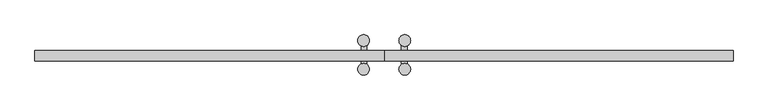
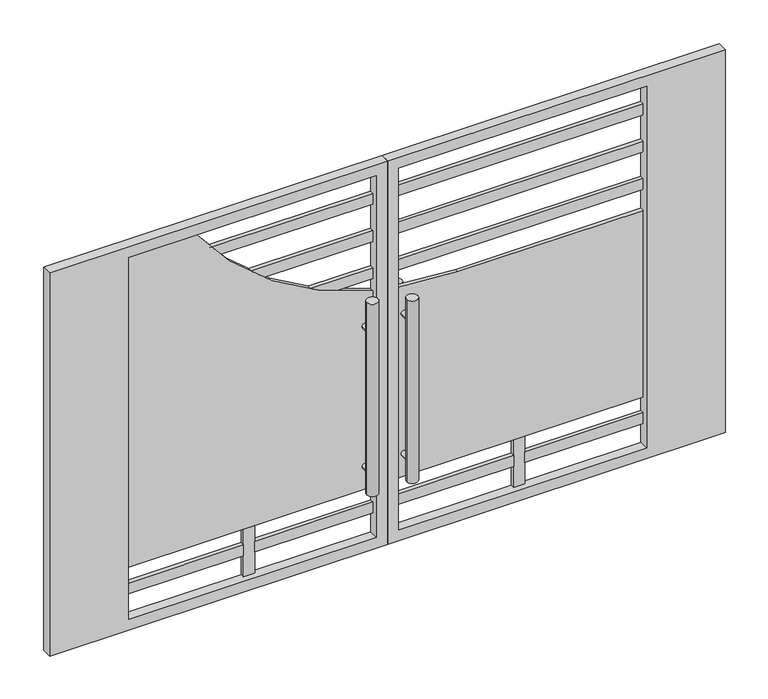
"""IFC4 building model written with IfcOpenShell, lengths in millimetres: proxy geometry."""

from ifc_helpers import new_model, si_unit, point, frame, frame_2d, origin, place, context, project, spatial, polyline, circle_curve, trimmed, segment, composite_curve, outline, extrude, source, transform, mapped, element, save


def generic_models_d903a639(model_context):
    return source(origin(), model_context, "Body", "SweptSolid", [
        extrude(outline(polyline([(0.0, -1524.918066), (0.0, 0.0), (1828.8, 0.0), (1828.8, -1524.918066), (0.0, -1524.918066)]), holes=[polyline([(50.8, -1168.4), (1778.0, -1168.4), (1778.0, -50.8), (50.8, -50.8), (50.8, -1168.4)])]), frame((0.0, -46.0617726, 0.0), z_axis=(0.0, 1.0, 0.0), x_axis=(0.0, 0.0, 1.0)), (0.0, 0.0, 1.0), 46.0617726),
        extrude(outline(polyline([(0.0, 1523.081934), (1828.8, 1523.081934), (1828.8, 0.0), (0.0, 0.0), (0.0, 1523.081934)]), holes=[polyline([(50.8, 1168.4), (50.8, 50.8), (1778.0, 50.8), (1778.0, 1168.4), (50.8, 1168.4)])]), frame((0.0, -46.0617726, 0.0), z_axis=(0.0, 1.0, 0.0), x_axis=(0.0, 0.0, 1.0)), (0.0, 0.0, 1.0), 46.0617726),
        extrude(outline(composite_curve([segment(polyline([(1778.0, -1168.4), (279.4, -1168.4), (279.4, -50.8), (1212.1744192, -50.8)]), True, "CONTINUOUS"), segment(trimmed(circle_curve(frame_2d((2582.6324877, 299.8877691)), 1414.6155764), [point((1212.1744192, -50.8))], [point((1778.0, -863.6))], True, "CARTESIAN"), True, "CONTINUOUS"), segment(polyline([(1778.0, -863.6), (1778.0, -1168.4)]), True, "CONTINUOUS")], self_intersect=False)), frame((0.0, -19.05, 0.0), z_axis=(0.0, 1.0, 0.0), x_axis=(0.0, 0.0, 1.0)), (0.0, 0.0, 1.0), 19.05),
        extrude(outline(composite_curve([segment(polyline([(279.4, 1168.4), (1168.4, 1168.4), (1168.4, 332.8073642)]), True, "CONTINUOUS"), segment(trimmed(circle_curve(frame_2d((2582.6324877, 299.8877691)), 1414.6155764), [point((1168.4, 332.8073642))], [point((1190.1194672, 50.8))], True, "CARTESIAN"), True, "CONTINUOUS"), segment(polyline([(1190.1194672, 50.8), (279.4, 50.8), (279.4, 1168.4)]), True, "CONTINUOUS")], self_intersect=False)), frame((0.0, -19.05, 0.0), z_axis=(0.0, 1.0, 0.0), x_axis=(0.0, 0.0, 1.0)), (0.0, 0.0, 1.0), 19.05),
        extrude(outline(composite_curve([segment(polyline([(1676.4, -50.8), (1676.4, -786.3350015)]), True, "CONTINUOUS"), segment(trimmed(circle_curve(frame_2d((2582.6324877, 299.8877691)), 1414.6155764), [point((1676.4, -786.3350015))], [point((1625.6, -741.8540639))], False, "CARTESIAN"), True, "CONTINUOUS"), segment(polyline([(1625.6, -741.8540639), (1625.6, -50.8), (1676.4, -50.8)]), True, "CONTINUOUS")], self_intersect=False)), frame((0.0, -19.05, 0.0), z_axis=(0.0, 1.0, 0.0), x_axis=(0.0, 0.0, 1.0)), (0.0, 0.0, 1.0), 19.05),
        extrude(outline(polyline([(1171.575, -19.05), (50.8, -19.05), (50.8, 0.0), (1171.575, 0.0), (1171.575, -19.05)])), frame((0.0, 0.0, 1625.6), z_axis=(0.0, 0.0, 1.0), x_axis=(1.0, 0.0, 0.0)), (0.0, 0.0, 1.0), 50.8),
        extrude(outline(composite_curve([segment(polyline([(1498.6, -50.8), (1498.6, -608.963591)]), True, "CONTINUOUS"), segment(trimmed(circle_curve(frame_2d((2582.6324877, 299.8877691)), 1414.6155764), [point((1498.6, -608.963591))], [point((1447.8, -544.6786605))], False, "CARTESIAN"), True, "CONTINUOUS"), segment(polyline([(1447.8, -544.6786605), (1447.8, -50.8), (1498.6, -50.8)]), True, "CONTINUOUS")], self_intersect=False)), frame((0.0, -19.05, 0.0), z_axis=(0.0, 1.0, 0.0), x_axis=(0.0, 0.0, 1.0)), (0.0, 0.0, 1.0), 19.05),
        extrude(outline(polyline([(1171.575, -19.05), (50.8, -19.05), (50.8, 0.0), (1171.575, 0.0), (1171.575, -19.05)])), frame((0.0, 0.0, 1447.8), z_axis=(0.0, 0.0, 1.0), x_axis=(1.0, 0.0, 0.0)), (0.0, 0.0, 1.0), 50.8),
        extrude(outline(composite_curve([segment(polyline([(1320.8, -50.8), (1320.8, -339.5776342)]), True, "CONTINUOUS"), segment(trimmed(circle_curve(frame_2d((2582.6324877, 299.8877691)), 1414.6155764), [point((1320.8, -339.5776342))], [point((1270.0, -227.4955652))], False, "CARTESIAN"), True, "CONTINUOUS"), segment(polyline([(1270.0, -227.4955652), (1270.0, -50.8), (1320.8, -50.8)]), True, "CONTINUOUS")], self_intersect=False)), frame((0.0, -19.05, 0.0), z_axis=(0.0, 1.0, 0.0), x_axis=(0.0, 0.0, 1.0)), (0.0, 0.0, 1.0), 19.05),
        extrude(outline(polyline([(1171.575, -19.05), (50.8, -19.05), (50.8, 0.0), (1171.575, 0.0), (1171.575, -19.05)])), frame((0.0, 0.0, 1270.0), z_axis=(0.0, 0.0, 1.0), x_axis=(1.0, 0.0, 0.0)), (0.0, 0.0, 1.0), 50.8),
        extrude(outline(polyline([(-635.0, -19.05), (-1168.4, -19.05), (-1168.4, 0.0), (-635.0, 0.0), (-635.0, -19.05)])), frame((0.0, 0.0, 152.4), z_axis=(0.0, 0.0, 1.0), x_axis=(1.0, 0.0, 0.0)), (0.0, 0.0, 1.0), 50.8),
        extrude(outline(polyline([(-50.8, -19.05), (-584.2, -19.05), (-584.2, 0.0), (-50.8, 0.0), (-50.8, -19.05)])), frame((0.0, 0.0, 152.4), z_axis=(0.0, 0.0, 1.0), x_axis=(1.0, 0.0, 0.0)), (0.0, 0.0, 1.0), 50.8),
        extrude(outline(polyline([(1168.4, -19.05), (635.0, -19.05), (635.0, 0.0), (1168.4, 0.0), (1168.4, -19.05)])), frame((0.0, 0.0, 152.4), z_axis=(0.0, 0.0, 1.0), x_axis=(1.0, 0.0, 0.0)), (0.0, 0.0, 1.0), 50.8),
        extrude(outline(polyline([(584.2, -19.05), (50.8, -19.05), (50.8, 0.0), (584.2, 0.0), (584.2, -19.05)])), frame((0.0, 0.0, 152.4), z_axis=(0.0, 0.0, 1.0), x_axis=(1.0, 0.0, 0.0)), (0.0, 0.0, 1.0), 50.8),
        extrude(outline(polyline([(-584.2, -19.05), (-635.0, -19.05), (-635.0, 0.0), (-584.2, 0.0), (-584.2, -19.05)])), frame((0.0, 0.0, 50.8), z_axis=(0.0, 0.0, 1.0), x_axis=(1.0, 0.0, 0.0)), (0.0, 0.0, 1.0), 228.6),
        extrude(outline(polyline([(635.0, -19.05), (584.2, -19.05), (584.2, 0.0), (635.0, 0.0), (635.0, -19.05)])), frame((0.0, 0.0, 50.8), z_axis=(0.0, 0.0, 1.0), x_axis=(1.0, 0.0, 0.0)), (0.0, 0.0, 1.0), 228.6),
        extrude(outline(composite_curve([segment(trimmed(circle_curve(frame_2d((-89.7949058, 43.7785099)), 25.4), [point((-64.3949058, 43.7785099))], [point((-115.1949058, 43.7785099))], False, "CARTESIAN"), True, "CONTINUOUS"), segment(trimmed(circle_curve(frame_2d((-89.7949058, 43.7785099)), 25.4), [point((-115.1949058, 43.7785099))], [point((-64.3949058, 43.7785099))], False, "CARTESIAN"), True, "CONTINUOUS")], self_intersect=False)), frame((0.0, 0.0, 279.4), z_axis=(0.0, 0.0, 1.0), x_axis=(1.0, 0.0, 0.0)), (0.0, 0.0, 1.0), 889.0),
        extrude(outline(composite_curve([segment(trimmed(circle_curve(frame_2d((89.7949058, 43.7785099)), 25.4), [point((64.3949058, 43.7785099))], [point((115.1949058, 43.7785099))], False, "CARTESIAN"), True, "CONTINUOUS"), segment(trimmed(circle_curve(frame_2d((89.7949058, 43.7785099)), 25.4), [point((115.1949058, 43.7785099))], [point((64.3949058, 43.7785099))], False, "CARTESIAN"), True, "CONTINUOUS")], self_intersect=False)), frame((0.0, 0.0, 279.4), z_axis=(0.0, 0.0, 1.0), x_axis=(1.0, 0.0, 0.0)), (0.0, 0.0, 1.0), 889.0),
        extrude(outline(composite_curve([segment(trimmed(circle_curve(frame_2d((-89.7949058, -81.8785099)), 25.4), [point((-64.3949058, -81.8785099))], [point((-115.1949058, -81.8785099))], False, "CARTESIAN"), True, "CONTINUOUS"), segment(trimmed(circle_curve(frame_2d((-89.7949058, -81.8785099)), 25.4), [point((-115.1949058, -81.8785099))], [point((-64.3949058, -81.8785099))], False, "CARTESIAN"), True, "CONTINUOUS")], self_intersect=False)), frame((0.0, 0.0, 298.8472671), z_axis=(0.0, 0.0, 1.0), x_axis=(1.0, 0.0, 0.0)), (0.0, 0.0, 1.0), 917.3073645),
        extrude(outline(composite_curve([segment(trimmed(circle_curve(frame_2d((89.7949058, -81.8785099)), 25.4), [point((64.3949058, -81.8785099))], [point((115.1949058, -81.8785099))], False, "CARTESIAN"), True, "CONTINUOUS"), segment(trimmed(circle_curve(frame_2d((89.7949058, -81.8785099)), 25.4), [point((115.1949058, -81.8785099))], [point((64.3949058, -81.8785099))], False, "CARTESIAN"), True, "CONTINUOUS")], self_intersect=False)), frame((0.0, 0.0, 298.8472671), z_axis=(0.0, 0.0, 1.0), x_axis=(1.0, 0.0, 0.0)), (0.0, 0.0, 1.0), 869.5527329),
        extrude(outline(composite_curve([segment(trimmed(circle_curve(frame_2d((1058.3458504, 88.119132)), 12.7), [point((1058.3458504, 75.419132))], [point((1058.3458504, 100.819132))], False, "CARTESIAN"), True, "CONTINUOUS"), segment(trimmed(circle_curve(frame_2d((1058.3458504, 88.119132)), 12.7), [point((1058.3458504, 100.819132))], [point((1058.3458504, 75.419132))], False, "CARTESIAN"), True, "CONTINUOUS")], self_intersect=False)), frame((0.0, -57.15, 0.0), z_axis=(0.0, 1.0, 0.0), x_axis=(0.0, 0.0, 1.0)), (0.0, 0.0, 1.0), 76.6172039),
        extrude(outline(composite_curve([segment(trimmed(circle_curve(frame_2d((389.4541496, 88.119132)), 12.7), [point((389.4541496, 75.419132))], [point((389.4541496, 100.819132))], False, "CARTESIAN"), True, "CONTINUOUS"), segment(trimmed(circle_curve(frame_2d((389.4541496, 88.119132)), 12.7), [point((389.4541496, 100.819132))], [point((389.4541496, 75.419132))], False, "CARTESIAN"), True, "CONTINUOUS")], self_intersect=False)), frame((0.0, -57.15, 0.0), z_axis=(0.0, 1.0, 0.0), x_axis=(0.0, 0.0, 1.0)), (0.0, 0.0, 1.0), 76.7981605),
        extrude(outline(composite_curve([segment(trimmed(circle_curve(frame_2d((1058.3458504, -88.119132)), 12.7), [point((1058.3458504, -75.419132))], [point((1058.3458504, -100.819132))], False, "CARTESIAN"), True, "CONTINUOUS"), segment(trimmed(circle_curve(frame_2d((1058.3458504, -88.119132)), 12.7), [point((1058.3458504, -100.819132))], [point((1058.3458504, -75.419132))], False, "CARTESIAN"), True, "CONTINUOUS")], self_intersect=False)), frame((0.0, -57.15, 0.0), z_axis=(0.0, 1.0, 0.0), x_axis=(0.0, 0.0, 1.0)), (0.0, 0.0, 1.0), 76.6172039),
        extrude(outline(composite_curve([segment(trimmed(circle_curve(frame_2d((389.4541496, -88.119132)), 12.7), [point((389.4541496, -75.419132))], [point((389.4541496, -100.819132))], False, "CARTESIAN"), True, "CONTINUOUS"), segment(trimmed(circle_curve(frame_2d((389.4541496, -88.119132)), 12.7), [point((389.4541496, -100.819132))], [point((389.4541496, -75.419132))], False, "CARTESIAN"), True, "CONTINUOUS")], self_intersect=False)), frame((0.0, -57.15, 0.0), z_axis=(0.0, 1.0, 0.0), x_axis=(0.0, 0.0, 1.0)), (0.0, 0.0, 1.0), 76.7981605),
    ])


if __name__ == "__main__":
    model = new_model("IFC4")
    model_context = context("Model", 3, world=origin())
    ifc_project = project(units=[si_unit("LENGTHUNIT", "METRE", prefix="MILLI")], contexts=[model_context])
    site = spatial("IfcSite", under=ifc_project)
    building = spatial("IfcBuilding", under=site)
    placement = place(None, origin())
    generic_models_shape = generic_models_d903a639(model_context)
    element("IfcBuildingElementProxy", 1, Name="Generic Models", at=placement, inside=building, context=model_context, shape_type="MappedRepresentation", body=[
        mapped(generic_models_shape, transform((0.0, 0.0, 0.0), x_axis=(1.0, 0.0, 0.0), y_axis=(0.0, 1.0, 0.0), z_axis=(0.0, 0.0, 1.0))),
    ])
    save(model, "model.ifc")

# Revit data of these elements
# Type
#   sheet = none
#   pipe = none
#   handal = none
#   faram = none
#   Default Elevation = 0
